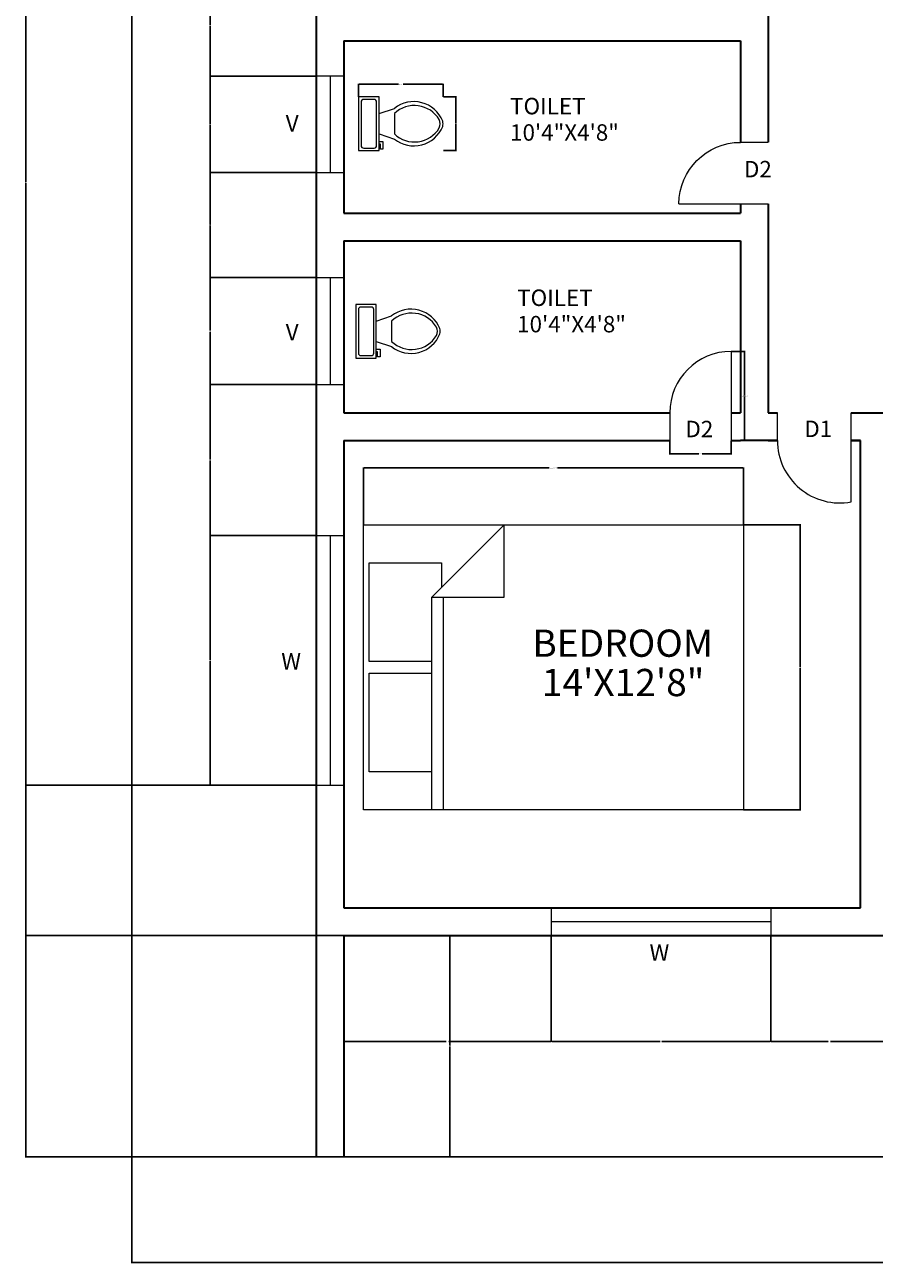
# Model space of a CAD drawing. Units: feet. Extents: x 1508 to 2265, y 1718 to 2421.
# Tile 1 of 4: x 1508 to 1784, y 1718 to 2121. Entities that reach past the tile are written whole.
import ezdxf

# ---------------------------------------------------------------- set-up
doc = ezdxf.new("R2010")
doc.units = ezdxf.units.FT
for name, color, linetype, lineweight in [('A-ANNO-DIMS', 2, 'Continuous', 18), ('A-ANNO-TEXT', 3, 'Continuous', 13), ('A-AREA-IDEN', 7, 'Continuous', 18), ('A-DOOR', 3, 'Continuous', 18), ('A-FLOR-FIXT', 9, 'Continuous', 18), ('A-FURN', 8, 'Continuous', 18), ('A-GLAZ', 4, 'Continuous', 18), ('A-WALL', 7, 'Continuous', 35), ('C-PROP', 7, 'Continuous', 25)]:
    doc.layers.add(name, color=color, linetype=linetype, lineweight=lineweight)
doc.styles.get("Standard").update_dxf_attribs({"font": 'arial.ttf'})
doc.dimstyles.get("Standard").update_dxf_attribs({"dimtxt": 0.18, "dimasz": 0.18, "dimexe": 0.18, "dimexo": 0.0625, "dimgap": 0.09, "dimtad": 0, "dimtih": 1, "dimtoh": 1, "dimdec": 4, "dimzin": 0, "dimdsep": 46, "dimtxsty": 'Standard', "dimcen": 0.09, "dimadec": 0, "dimazin": 0, "dimtfac": 1, "dimtdec": 4, "dimtofl": 0, "dimtmove": 0, "dimatfit": 3, "dimfxl": 1, "dimtolj": 1, "dimtzin": 0, "dimarcsym": 0})

# ---------------------------------------------------------------- blocks, each defined once
blk = doc.blocks.new('Toilet - top')
for p, q in [((9.5, -6), (9.5, -2)), ((-10, -8.5), (-8, -8.5)), ((-10, -9.5), (-10, -8.5)), ((-7, -9.5), (-10, -9.5)), ((-8, -8.5), (-8, -8)), ((-7, -8), (-7, -9.5)), ((-4, -8), (-6, -14)), ((4, -8), (6, -14)), ((4, -14), (-4, -14))]:
    blk.add_line(p, q)
blk.add_lwpolyline([(10.5, -8), (10.5, 0), (-10.5, 0), (-10.5, -8)], close=True)
for points in [[(-9.5, -2), (-9.5, -6)], [(8.5, -1), (-8.5, -1)], [(-8.5, -7), (8.5, -7)]]:
    blk.add_lwpolyline(points)
for centre, radius, start, end in [((-8.62, -1.88), 0.884, 81.8699, 188.1301), ((8.62, -1.88), 0.884, 351.8699, 98.1301), ((-8.62, -6.12), 0.884, 171.8699, 278.1301), ((8.62, -6.12), 0.884, 261.8699, 8.1301), ((3.52, -21.58), 12.17, 141.4691, 247.9714), ((4.2, -21.82), 11.33, 136.3677, 238.9468), ((-3.52, -21.58), 12.17, 292.0284, 38.5307), ((-4.2, -21.82), 11.33, 301.053, 43.6321), ((0, -27.88), 4, 245.7318, 294.2682), ((0, -29), 4, 254.8605, 285.1395)]:
    blk.add_arc(centre, radius, start, end)
blk = doc.blocks.new('Bed - Queen')
for p, q in [((0, -80.00003), (0, 0)), ((0, 0), (59.99999, 0)), ((59.99999, 0), (59.99999, -80.00003)), ((7.99999, -1.2), (28.79998, -1.2)), ((7.99999, -14.4), (7.99999, -1.2)), ((28.79998, -1.2), (28.79998, -14.4)), ((31.19999, -1.2), (51.99999, -1.2)), ((31.19999, -14.4), (31.19999, -1.2)), ((51.99999, -1.2), (51.99999, -16.4)), ((0, -14.4), (44.8, -14.4)), ((59.99999, -29.6), (44.8, -14.4)), ((44.8, -14.4), (44.8, -29.6)), ((44.8, -16.8), (0, -16.8)), ((51.99999, -16.4), (46.79936, -16.4)), ((44.8, -29.6), (59.99999, -29.6)), ((59.99999, -80.00003), (0, -80.00003))]:
    blk.add_line(p, q)
blk = doc.blocks.new('DOOR-LEAF-20')
blk.add_line((20, 29), (20, 0))
blk.add_arc((20, 9), 20, 90, 180)
blk = doc.blocks.new('*D13')
at = {"layer": 'A-ANNO-DIMS', "color": 0, "lineweight": -2, "transparency": 16777216}
for p, q in [((1737.87, 2014.26), (1742.33, 2014.26)), ((1742.15, 2014.08), (1742.15, 1999.94)), ((1742.15, 1985.44), (1742.15, 1999.58)), ((1737.87, 1985.26), (1742.33, 1985.26))]:
    blk.add_line(p, q, dxfattribs=at)
at = {"layer": 'A-ANNO-DIMS', "color": 0, "transparency": 16777216}
for points in [[(1742.12, 2014.08), (1742.18, 2014.08), (1742.15, 2014.26)], [(1742.12, 1985.44), (1742.18, 1985.44), (1742.15, 1985.26)]]:
    blk.add_solid(points, dxfattribs=at)
at = {"layer": 'Defpoints', "color": 0, "transparency": 16777216}
for p in [(1737.8, 2014.26), (1742.15, 2014.26), (1737.8, 1985.26)]:
    blk.add_point(p, dxfattribs=at)
at = {"layer": 'A-ANNO-DIMS', "color": 0, "transparency": 16777216, "insert": (1742.15, 1999.76), "char_height": 0.18, "attachment_point": 5}
blk.add_mtext('\\A1;D2 SWING 29 TYP.', dxfattribs=at)
blk = doc.blocks.new('*D14')
at = {"layer": 'A-ANNO-DIMS', "color": 0, "lineweight": -2, "transparency": 16777216}
for p, q in [((1717.8, 1985.2), (1717.8, 1980.73)), ((1737.8, 1985.2), (1737.8, 1980.73)), ((1717.98, 1980.91), (1727.28, 1980.91)), ((1737.62, 1980.91), (1728.33, 1980.91))]:
    blk.add_line(p, q, dxfattribs=at)
at = {"layer": 'A-ANNO-DIMS', "color": 0, "transparency": 16777216}
for points in [[(1717.98, 1980.94), (1717.98, 1980.88), (1717.8, 1980.91)], [(1737.62, 1980.94), (1737.62, 1980.88), (1737.8, 1980.91)]]:
    blk.add_solid(points, dxfattribs=at)
at = {"layer": 'Defpoints', "color": 0, "transparency": 16777216}
for p in [(1717.8, 1985.26), (1737.8, 1985.26), (1737.8, 1980.91)]:
    blk.add_point(p, dxfattribs=at)
at = {"layer": 'A-ANNO-DIMS', "color": 0, "transparency": 16777216, "insert": (1727.8, 1980.91), "char_height": 0.18, "attachment_point": 5}
blk.add_mtext('\\A1;20 TYP.', dxfattribs=at)
blk = doc.blocks.new('*D15')
at = {"layer": 'A-ANNO-DIMS', "color": 0, "lineweight": -2, "transparency": 16777216}
for p, q in [((1618.2, 1957.86), (1618.2, 1976.51)), ((1618.38, 1976.33), (1678.59, 1976.33)), ((1741.56, 1976.33), (1681.34, 1976.33)), ((1741.74, 1957.86), (1741.74, 1976.51))]:
    blk.add_line(p, q, dxfattribs=at)
at = {"layer": 'A-ANNO-DIMS', "color": 0, "transparency": 16777216}
for points in [[(1618.38, 1976.36), (1618.38, 1976.3), (1618.2, 1976.33)], [(1741.56, 1976.36), (1741.56, 1976.3), (1741.74, 1976.33)]]:
    blk.add_solid(points, dxfattribs=at)
at = {"layer": 'Defpoints', "color": 0, "transparency": 16777216}
for p in [(1618.2, 1976.33), (1618.2, 1957.8), (1741.74, 1957.8)]:
    blk.add_point(p, dxfattribs=at)
at = {"layer": 'A-ANNO-DIMS', "color": 0, "transparency": 16777216, "insert": (1679.97, 1976.33), "char_height": 0.18, "attachment_point": 5}
blk.add_mtext('\\A1;QUEEN BED 124 TYP.', dxfattribs=at)
blk = doc.blocks.new('*D16')
at = {"layer": 'A-ANNO-DIMS', "color": 0, "lineweight": -2, "transparency": 16777216}
for p, q in [((1741.8, 1957.8), (1760.45, 1957.8)), ((1760.27, 1957.62), (1760.27, 1911.65)), ((1760.27, 1865.32), (1760.27, 1911.29)), ((1741.8, 1865.14), (1760.45, 1865.14))]:
    blk.add_line(p, q, dxfattribs=at)
at = {"layer": 'A-ANNO-DIMS', "color": 0, "transparency": 16777216}
for points in [[(1760.24, 1957.62), (1760.3, 1957.62), (1760.27, 1957.8)], [(1760.24, 1865.32), (1760.3, 1865.32), (1760.27, 1865.14)]]:
    blk.add_solid(points, dxfattribs=at)
at = {"layer": 'Defpoints', "color": 0, "transparency": 16777216}
for p in [(1741.74, 1957.8), (1760.27, 1957.8), (1741.74, 1865.14)]:
    blk.add_point(p, dxfattribs=at)
at = {"layer": 'A-ANNO-DIMS', "color": 0, "transparency": 16777216, "insert": (1760.27, 1911.47), "char_height": 0.18, "attachment_point": 5}
blk.add_mtext('\\A1;93 TYP.', dxfattribs=at)
blk = doc.blocks.new('*D17')
at = {"layer": 'A-ANNO-DIMS', "color": 0, "lineweight": -2, "transparency": 16777216}
for p, q in [((1616.62, 2097.09), (1616.62, 2101.33)), ((1616.8, 2101.15), (1629.58, 2101.15)), ((1643.92, 2101.15), (1631.14, 2101.15)), ((1644.1, 2097.09), (1644.1, 2101.33))]:
    blk.add_line(p, q, dxfattribs=at)
at = {"layer": 'A-ANNO-DIMS', "color": 0, "transparency": 16777216}
for points in [[(1616.8, 2101.18), (1616.8, 2101.12), (1616.62, 2101.15)], [(1643.92, 2101.18), (1643.92, 2101.12), (1644.1, 2101.15)]]:
    blk.add_solid(points, dxfattribs=at)
at = {"layer": 'Defpoints', "color": 0, "transparency": 16777216}
for p in [(1616.62, 2101.15), (1616.62, 2097.03), (1644.1, 2097.03)]:
    blk.add_point(p, dxfattribs=at)
at = {"layer": 'A-ANNO-DIMS', "color": 0, "transparency": 16777216, "insert": (1630.36, 2101.15), "char_height": 0.18, "attachment_point": 5}
blk.add_mtext('\\A1;WC 27 TYP.', dxfattribs=at)
blk = doc.blocks.new('*D18')
at = {"layer": 'A-ANNO-DIMS', "color": 0, "lineweight": -2, "transparency": 16777216}
for p, q in [((1644.16, 2097.03), (1648.4, 2097.03)), ((1648.22, 2096.85), (1648.22, 2088.48)), ((1648.22, 2079.75), (1648.22, 2088.12)), ((1644.16, 2079.57), (1648.4, 2079.57))]:
    blk.add_line(p, q, dxfattribs=at)
at = {"layer": 'A-ANNO-DIMS', "color": 0, "transparency": 16777216}
for points in [[(1648.19, 2096.85), (1648.25, 2096.85), (1648.22, 2097.03)], [(1648.19, 2079.75), (1648.25, 2079.75), (1648.22, 2079.57)]]:
    blk.add_solid(points, dxfattribs=at)
at = {"layer": 'Defpoints', "color": 0, "transparency": 16777216}
for p in [(1644.1, 2097.03), (1648.22, 2097.03), (1644.1, 2079.57)]:
    blk.add_point(p, dxfattribs=at)
at = {"layer": 'A-ANNO-DIMS', "color": 0, "transparency": 16777216, "insert": (1648.22, 2088.3), "char_height": 0.18, "attachment_point": 5}
blk.add_mtext('\\A1;17 TYP.', dxfattribs=at)
blk = doc.blocks.new('*D31')
at = {"layer": 'A-ANNO-DIMS', "color": 0, "lineweight": -2, "transparency": 16777216}
for p, q in [((1542.8, 1752.2), (1542.8, 1717.61)), ((2230.8, 1752.2), (2230.8, 1717.61)), ((1542.98, 1717.79), (1886.52, 1717.79)), ((2230.62, 1717.79), (1887.09, 1717.79))]:
    blk.add_line(p, q, dxfattribs=at)
at = {"layer": 'A-ANNO-DIMS', "color": 0, "transparency": 16777216}
for points in [[(1542.98, 1717.82), (1542.98, 1717.76), (1542.8, 1717.79)], [(2230.62, 1717.82), (2230.62, 1717.76), (2230.8, 1717.79)]]:
    blk.add_solid(points, dxfattribs=at)
at = {"layer": 'Defpoints', "color": 0, "transparency": 16777216}
for p in [(1542.8, 1752.26), (2230.8, 1752.26), (2230.8, 1717.79)]:
    blk.add_point(p, dxfattribs=at)
at = {"layer": 'A-ANNO-DIMS', "color": 0, "transparency": 16777216, "insert": (1886.8, 1717.79), "char_height": 0.18, "attachment_point": 5}
blk.add_mtext('\\A1;688', dxfattribs=at)
blk = doc.blocks.new('*D32')
at = {"layer": 'A-ANNO-DIMS', "color": 0, "lineweight": -2, "transparency": 16777216}
for p, q in [((1542.74, 2386.26), (1508.15, 2386.26)), ((1508.33, 2386.08), (1508.33, 2069.44)), ((1508.33, 1752.44), (1508.33, 2069.08)), ((1542.74, 1752.26), (1508.15, 1752.26))]:
    blk.add_line(p, q, dxfattribs=at)
at = {"layer": 'A-ANNO-DIMS', "color": 0, "transparency": 16777216}
for points in [[(1508.3, 2386.08), (1508.36, 2386.08), (1508.33, 2386.26)], [(1508.3, 1752.44), (1508.36, 1752.44), (1508.33, 1752.26)]]:
    blk.add_solid(points, dxfattribs=at)
at = {"layer": 'Defpoints', "color": 0, "transparency": 16777216}
for p in [(1508.33, 2386.26), (1542.8, 2386.26), (1542.8, 1752.26)]:
    blk.add_point(p, dxfattribs=at)
at = {"layer": 'A-ANNO-DIMS', "color": 0, "transparency": 16777216, "insert": (1508.33, 2069.26), "char_height": 0.18, "attachment_point": 5}
blk.add_mtext('\\A1;634', dxfattribs=at)
blk = doc.blocks.new('*D35')
at = {"layer": 'A-ANNO-DIMS', "color": 0, "lineweight": -2, "transparency": 16777216}
for p, q in [((1611.87, 1824.26), (1646.46, 1824.26)), ((1646.28, 1824.08), (1646.28, 1788.44)), ((1646.28, 1752.44), (1646.28, 1788.08)), ((1611.87, 1752.26), (1646.46, 1752.26))]:
    blk.add_line(p, q, dxfattribs=at)
at = {"layer": 'A-ANNO-DIMS', "color": 0, "transparency": 16777216}
for points in [[(1646.25, 1824.08), (1646.31, 1824.08), (1646.28, 1824.26)], [(1646.25, 1752.44), (1646.31, 1752.44), (1646.28, 1752.26)]]:
    blk.add_solid(points, dxfattribs=at)
at = {"layer": 'Defpoints', "color": 0, "transparency": 16777216}
for p in [(1611.8, 1824.26), (1611.8, 1752.26), (1646.28, 1752.26)]:
    blk.add_point(p, dxfattribs=at)
at = {"layer": 'A-ANNO-DIMS', "color": 0, "transparency": 16777216, "insert": (1646.28, 1788.26), "char_height": 0.18, "attachment_point": 5}
blk.add_mtext('\\A1;72', dxfattribs=at)
blk = doc.blocks.new('*D53')
at = {"layer": 'A-ANNO-DIMS', "color": 0, "lineweight": -2, "transparency": 16777216}
for p, q in [((1602.74, 1873.09), (1508.15, 1873.09)), ((1508.33, 1872.91), (1508.33, 1848.86)), ((1508.33, 1824.44), (1508.33, 1848.49)), ((1611.74, 1824.26), (1508.15, 1824.26))]:
    blk.add_line(p, q, dxfattribs=at)
at = {"layer": 'A-ANNO-DIMS', "color": 0, "transparency": 16777216}
for points in [[(1508.3, 1872.91), (1508.36, 1872.91), (1508.33, 1873.09)], [(1508.3, 1824.44), (1508.36, 1824.44), (1508.33, 1824.26)]]:
    blk.add_solid(points, dxfattribs=at)
at = {"layer": 'Defpoints', "color": 0, "transparency": 16777216}
for p in [(1508.33, 1873.09), (1602.8, 1873.09), (1611.8, 1824.26)]:
    blk.add_point(p, dxfattribs=at)
at = {"layer": 'A-ANNO-DIMS', "color": 0, "transparency": 16777216, "insert": (1508.33, 1848.67), "char_height": 0.18, "attachment_point": 5}
blk.add_mtext('\\A1;48.83', dxfattribs=at)
blk = doc.blocks.new('*D54')
at = {"layer": 'A-ANNO-DIMS', "color": 0, "lineweight": -2, "transparency": 16777216}
for p, q in [((1602.74, 1954.4), (1568.15, 1954.4)), ((1568.33, 1954.22), (1568.33, 1913.93)), ((1568.33, 1873.27), (1568.33, 1913.56)), ((1602.74, 1873.09), (1568.15, 1873.09))]:
    blk.add_line(p, q, dxfattribs=at)
at = {"layer": 'A-ANNO-DIMS', "color": 0, "transparency": 16777216}
for points in [[(1568.3, 1954.22), (1568.36, 1954.22), (1568.33, 1954.4)], [(1568.3, 1873.27), (1568.36, 1873.27), (1568.33, 1873.09)]]:
    blk.add_solid(points, dxfattribs=at)
at = {"layer": 'Defpoints', "color": 0, "transparency": 16777216}
for p in [(1568.33, 1954.4), (1602.8, 1954.4), (1602.8, 1873.09)]:
    blk.add_point(p, dxfattribs=at)
at = {"layer": 'A-ANNO-DIMS', "color": 0, "transparency": 16777216, "insert": (1568.33, 1913.75), "char_height": 0.18, "attachment_point": 5}
blk.add_mtext('\\A1;81.32', dxfattribs=at)
blk = doc.blocks.new('*D55')
at = {"layer": 'A-ANNO-DIMS', "color": 0, "lineweight": -2, "transparency": 16777216}
for p, q in [((1602.74, 2003.44), (1568.15, 2003.44)), ((1568.33, 2003.26), (1568.33, 1979.11)), ((1568.33, 1954.58), (1568.33, 1978.74)), ((1602.74, 1954.4), (1568.15, 1954.4))]:
    blk.add_line(p, q, dxfattribs=at)
at = {"layer": 'A-ANNO-DIMS', "color": 0, "transparency": 16777216}
for points in [[(1568.3, 2003.26), (1568.36, 2003.26), (1568.33, 2003.44)], [(1568.3, 1954.58), (1568.36, 1954.58), (1568.33, 1954.4)]]:
    blk.add_solid(points, dxfattribs=at)
at = {"layer": 'Defpoints', "color": 0, "transparency": 16777216}
for p in [(1568.33, 2003.44), (1602.8, 2003.44), (1602.8, 1954.4)]:
    blk.add_point(p, dxfattribs=at)
at = {"layer": 'A-ANNO-DIMS', "color": 0, "transparency": 16777216, "insert": (1568.33, 1978.92), "char_height": 0.18, "attachment_point": 5}
blk.add_mtext('\\A1;49.04', dxfattribs=at)
blk = doc.blocks.new('*D56')
at = {"layer": 'A-ANNO-DIMS', "color": 0, "lineweight": -2, "transparency": 16777216}
for p, q in [((1602.74, 2038.25), (1568.15, 2038.25)), ((1568.33, 2038.07), (1568.33, 2021.03)), ((1568.33, 2003.62), (1568.33, 2020.66)), ((1602.74, 2003.44), (1568.15, 2003.44))]:
    blk.add_line(p, q, dxfattribs=at)
at = {"layer": 'A-ANNO-DIMS', "color": 0, "transparency": 16777216}
for points in [[(1568.3, 2038.07), (1568.36, 2038.07), (1568.33, 2038.25)], [(1568.3, 2003.62), (1568.36, 2003.62), (1568.33, 2003.44)]]:
    blk.add_solid(points, dxfattribs=at)
at = {"layer": 'Defpoints', "color": 0, "transparency": 16777216}
for p in [(1568.33, 2038.25), (1602.8, 2038.25), (1602.8, 2003.44)]:
    blk.add_point(p, dxfattribs=at)
at = {"layer": 'A-ANNO-DIMS', "color": 0, "transparency": 16777216, "insert": (1568.33, 2020.84), "char_height": 0.18, "attachment_point": 5}
blk.add_mtext('\\A1;34.804', dxfattribs=at)
blk = doc.blocks.new('*D57')
at = {"layer": 'A-ANNO-DIMS', "color": 0, "lineweight": -2, "transparency": 16777216}
for p, q in [((1602.74, 2072.43), (1568.15, 2072.43)), ((1568.33, 2072.25), (1568.33, 2055.52)), ((1568.33, 2038.43), (1568.33, 2055.16)), ((1602.74, 2038.25), (1568.15, 2038.25))]:
    blk.add_line(p, q, dxfattribs=at)
at = {"layer": 'A-ANNO-DIMS', "color": 0, "transparency": 16777216}
for points in [[(1568.3, 2072.25), (1568.36, 2072.25), (1568.33, 2072.43)], [(1568.3, 2038.43), (1568.36, 2038.43), (1568.33, 2038.25)]]:
    blk.add_solid(points, dxfattribs=at)
at = {"layer": 'Defpoints', "color": 0, "transparency": 16777216}
for p in [(1568.33, 2072.43), (1602.8, 2072.43), (1602.8, 2038.25)]:
    blk.add_point(p, dxfattribs=at)
at = {"layer": 'A-ANNO-DIMS', "color": 0, "transparency": 16777216, "insert": (1568.33, 2055.34), "char_height": 0.18, "attachment_point": 5}
blk.add_mtext('\\A1;34.19', dxfattribs=at)
blk = doc.blocks.new('*D58')
at = {"layer": 'A-ANNO-DIMS', "color": 0, "lineweight": -2, "transparency": 16777216}
for p, q in [((1602.74, 2103.84), (1568.15, 2103.84)), ((1568.33, 2103.66), (1568.33, 2088.32)), ((1568.33, 2072.61), (1568.33, 2087.96)), ((1602.74, 2072.43), (1568.15, 2072.43))]:
    blk.add_line(p, q, dxfattribs=at)
at = {"layer": 'A-ANNO-DIMS', "color": 0, "transparency": 16777216}
for points in [[(1568.3, 2103.66), (1568.36, 2103.66), (1568.33, 2103.84)], [(1568.3, 2072.61), (1568.36, 2072.61), (1568.33, 2072.43)]]:
    blk.add_solid(points, dxfattribs=at)
at = {"layer": 'Defpoints', "color": 0, "transparency": 16777216}
for p in [(1568.33, 2103.84), (1602.8, 2103.84), (1602.8, 2072.43)]:
    blk.add_point(p, dxfattribs=at)
at = {"layer": 'A-ANNO-DIMS', "color": 0, "transparency": 16777216, "insert": (1568.33, 2088.14), "char_height": 0.18, "attachment_point": 5}
blk.add_mtext('\\A1;31.41', dxfattribs=at)
blk = doc.blocks.new('*D59')
at = {"layer": 'A-ANNO-DIMS', "color": 0, "lineweight": -2, "transparency": 16777216}
for p, q in [((1602.74, 2136.59), (1568.15, 2136.59)), ((1568.33, 2136.41), (1568.33, 2120.4)), ((1568.33, 2104.02), (1568.33, 2120.03)), ((1602.74, 2103.84), (1568.15, 2103.84))]:
    blk.add_line(p, q, dxfattribs=at)
at = {"layer": 'A-ANNO-DIMS', "color": 0, "transparency": 16777216}
for points in [[(1568.3, 2136.41), (1568.36, 2136.41), (1568.33, 2136.59)], [(1568.3, 2104.02), (1568.36, 2104.02), (1568.33, 2103.84)]]:
    blk.add_solid(points, dxfattribs=at)
at = {"layer": 'Defpoints', "color": 0, "transparency": 16777216}
for p in [(1568.33, 2136.59), (1602.8, 2136.59), (1602.8, 2103.84)]:
    blk.add_point(p, dxfattribs=at)
at = {"layer": 'A-ANNO-DIMS', "color": 0, "transparency": 16777216, "insert": (1568.33, 2120.22), "char_height": 0.18, "attachment_point": 5}
blk.add_mtext('\\A1;32.74', dxfattribs=at)
blk = doc.blocks.new('*D66')
at = {"layer": 'A-ANNO-DIMS', "color": 0, "lineweight": -2, "transparency": 16777216}
for p, q in [((1611.8, 1824.2), (1611.8, 1789.61)), ((1679.25, 1824.2), (1679.25, 1789.61)), ((1611.98, 1789.79), (1645.13, 1789.79)), ((1679.07, 1789.79), (1645.92, 1789.79))]:
    blk.add_line(p, q, dxfattribs=at)
at = {"layer": 'A-ANNO-DIMS', "color": 0, "transparency": 16777216}
for points in [[(1611.98, 1789.82), (1611.98, 1789.76), (1611.8, 1789.79)], [(1679.07, 1789.82), (1679.07, 1789.76), (1679.25, 1789.79)]]:
    blk.add_solid(points, dxfattribs=at)
at = {"layer": 'Defpoints', "color": 0, "transparency": 16777216}
for p in [(1611.8, 1824.26), (1679.25, 1824.26), (1611.8, 1789.79)]:
    blk.add_point(p, dxfattribs=at)
at = {"layer": 'A-ANNO-DIMS', "color": 0, "transparency": 16777216, "insert": (1645.53, 1789.79), "char_height": 0.18, "attachment_point": 5}
blk.add_mtext('\\A1;67.45', dxfattribs=at)
blk = doc.blocks.new('*D67')
at = {"layer": 'A-ANNO-DIMS', "color": 0, "lineweight": -2, "transparency": 16777216}
for p, q in [((1679.25, 1824.2), (1679.25, 1789.61)), ((1750.65, 1824.2), (1750.65, 1789.61)), ((1679.43, 1789.79), (1714.63, 1789.79)), ((1750.47, 1789.79), (1715.27, 1789.79))]:
    blk.add_line(p, q, dxfattribs=at)
at = {"layer": 'A-ANNO-DIMS', "color": 0, "transparency": 16777216}
for points in [[(1679.43, 1789.82), (1679.43, 1789.76), (1679.25, 1789.79)], [(1750.47, 1789.82), (1750.47, 1789.76), (1750.65, 1789.79)]]:
    blk.add_solid(points, dxfattribs=at)
at = {"layer": 'Defpoints', "color": 0, "transparency": 16777216}
for p in [(1679.25, 1824.26), (1750.65, 1824.26), (1679.25, 1789.79)]:
    blk.add_point(p, dxfattribs=at)
at = {"layer": 'A-ANNO-DIMS', "color": 0, "transparency": 16777216, "insert": (1714.95, 1789.79), "char_height": 0.18, "attachment_point": 5}
blk.add_mtext('\\A1;71.4', dxfattribs=at)
blk = doc.blocks.new('*D68')
at = {"layer": 'A-ANNO-DIMS', "color": 0, "lineweight": -2, "transparency": 16777216}
for p, q in [((1750.65, 1824.2), (1750.65, 1789.61)), ((1788.8, 1824.2), (1788.8, 1789.61)), ((1750.83, 1789.79), (1769.33, 1789.79)), ((1788.62, 1789.79), (1770.12, 1789.79))]:
    blk.add_line(p, q, dxfattribs=at)
at = {"layer": 'A-ANNO-DIMS', "color": 0, "transparency": 16777216}
for points in [[(1750.83, 1789.82), (1750.83, 1789.76), (1750.65, 1789.79)], [(1788.62, 1789.82), (1788.62, 1789.76), (1788.8, 1789.79)]]:
    blk.add_solid(points, dxfattribs=at)
at = {"layer": 'Defpoints', "color": 0, "transparency": 16777216}
for p in [(1750.65, 1824.26), (1788.8, 1824.26), (1750.65, 1789.79)]:
    blk.add_point(p, dxfattribs=at)
at = {"layer": 'A-ANNO-DIMS', "color": 0, "transparency": 16777216, "insert": (1769.73, 1789.79), "char_height": 0.18, "attachment_point": 5}
blk.add_mtext('\\A1;38.15', dxfattribs=at)

msp = doc.modelspace()

# ---------------------------------------------------------------- linework, layer by layer
at = {"layer": 'A-DOOR'}
for p, q in [((1740.8049, 2082.2608), (1749.8049, 2082.2608)), ((1717.8049, 1994.2608), (1717.8049, 1985.2608)), ((1752.8049, 1985.2608), (1752.8049, 1994.2608)), ((1776.8049, 1965.2608), (1776.8049, 1994.2608))]:
    msp.add_line(p, q, dxfattribs=at)
msp.add_arc((1773.1382, 1985.2608), 20.3333, 180, 280.388858, dxfattribs=at)
at = {"layer": 'A-GLAZ'}
for p, q in [((1602.8049, 2103.8448), (1611.8049, 2103.8448)), ((1607.3049, 2103.8448), (1607.3049, 2072.4348)), ((1602.8049, 2072.4348), (1611.8049, 2072.4348)), ((1602.8049, 2038.2467), (1611.8049, 2038.2467)), ((1607.3049, 2038.2467), (1607.3049, 2003.4426)), ((1602.8049, 2003.4426), (1611.8049, 2003.4426)), ((1602.8049, 1954.4046), (1611.8049, 1954.4046)), ((1607.3049, 1954.4046), (1607.3049, 1873.0878)), ((1602.8049, 1873.0878), (1611.8049, 1873.0878)), ((1679.2508, 1833.2608), (1679.2508, 1824.2608)), ((1750.6528, 1833.2608), (1750.6528, 1824.2608)), ((1679.2508, 1828.7608), (1750.6528, 1828.7608))]:
    msp.add_line(p, q, dxfattribs=at)
at = {"layer": 'A-WALL'}
for p, q in [((1602.8049, 2192.2608), (1602.8049, 1752.2608)), ((1749.8049, 2189.2608), (1749.8049, 2082.2608)), ((1602.8049, 2115.2608), (1602.8049, 2059.2608)), ((1611.8049, 2115.2608), (1740.8049, 2115.2608)), ((1611.8049, 2115.2608), (1611.8049, 2059.2608)), ((1680.8049, 2115.2608), (1740.8049, 2115.2608)), ((1740.8049, 2115.2608), (1740.8049, 2082.2608)), ((1611.8049, 2059.2608), (1740.8049, 2059.2608)), ((1740.8049, 2062.2608), (1740.8049, 2059.2608)), ((1749.8049, 2062.2608), (1749.8049, 1994.2608)), ((1602.8049, 2050.2608), (1602.8049, 1994.2608)), ((1611.8049, 2050.2608), (1740.8049, 2050.2608)), ((1611.8049, 2050.2608), (1611.8049, 1994.2608)), ((1740.8049, 2050.2608), (1740.8049, 1994.2608)), ((1611.8049, 1994.2608), (1717.8049, 1994.2608)), ((1737.8049, 1994.2608), (1740.8049, 1994.2608)), ((1749.8049, 1994.2608), (1752.8049, 1994.2608)), ((1776.8049, 1994.2608), (1791.8049, 1994.2608)), ((1602.8049, 1985.2608), (1602.8049, 1752.2608)), ((1611.8049, 1985.2608), (1717.8049, 1985.2608)), ((1611.8049, 1985.2608), (1611.8049, 1833.2608)), ((1737.8049, 1985.2608), (1740.8049, 1985.2608)), ((1752.8049, 1985.2608), (1740.8049, 1985.2608)), ((1749.8049, 1985.2608), (1752.8049, 1985.2608)), ((1779.8049, 1985.2608), (1776.8049, 1985.2608)), ((1776.8049, 1985.2608), (1779.8049, 1985.2608)), ((1779.8049, 1833.2608), (1779.8049, 1985.2608)), ((1611.8049, 1833.2608), (1779.8049, 1833.2608)), ((1611.8049, 1824.2608), (1974.8049, 1824.2608)), ((1611.8049, 1824.2608), (1611.8049, 1752.2608))]:
    msp.add_line(p, q, dxfattribs=at)
at = {"layer": 'C-PROP'}
for p, q in [((1542.8049, 2386.2608), (1542.8049, 1752.2608)), ((1602.8049, 1752.2608), (1542.8049, 1752.2608)), ((1611.8049, 1752.2608), (1602.8049, 1752.2608)), ((1611.8049, 1752.2608), (2230.8049, 1752.2608))]:
    msp.add_line(p, q, dxfattribs=at)

# ---------------------------------------------------------------- block references
at = {"layer": 'A-DOOR', "extrusion": (0, 0, -1), "zscale": -1, "rotation": 270.0000000000007}
msp.add_blockref('DOOR-LEAF-20', (-1749.8046, 2082.2606), dxfattribs=at)
at = {"layer": 'A-DOOR'}
msp.add_blockref('DOOR-LEAF-20', (1717.805, 1985.261), dxfattribs=at)
at = {"layer": 'A-FLOR-FIXT', "xscale": 0.8315942650714294, "yscale": 0.8315942650714294, "zscale": 0.8315942650714294, "rotation": 90}
for p in [(1616.6188, 2088.2998), (1615.7002, 2020.784)]:
    msp.add_blockref('Toilet - top', p, dxfattribs=at)
at = {"layer": 'A-FURN', "xscale": 1.544203597856591, "yscale": 1.544203597856591, "zscale": 1.544203597856591, "rotation": 90}
msp.add_blockref('Bed - Queen', (1618.1998, 1865.1449), dxfattribs=at)

# ---------------------------------------------------------------- texts
at = {"layer": 'A-ANNO-TEXT'}
for s, height, p in [('V', 5.3453, (1592.8942, 2085.7633)), ('D2', 5.34528, (1741.9372, 2070.8617)), ('V', 5.3453, (1592.8942, 2017.8526)), ('D2', 5.34528, (1722.8941, 1986.3233)), ('D1', 5.34528, (1761.5653, 1986.3768)), ('W', 5.3453, (1591.4512, 1910.7582)), ('W', 5.3453, (1711.2296, 1815.9883))]:
    msp.add_text(s, height=height, dxfattribs=at).set_placement(p)
at = {"layer": 'A-AREA-IDEN'}
for s, height, p in [('TOILET', 5.34528, (1665.8694, 2091.3765)), ('10\'4"X4\'8"', 5.34528, (1665.8694, 2082.7898)), ('TOILET', 5.34528, (1668.1636, 2029.0268)), ('10\'4"X4\'8"', 5.34528, (1668.1636, 2020.4401)), ('BEDROOM', 8.85057, (1673.1135, 1914.8931)), ('14\'X12\'8"', 8.85057, (1676.1992, 1902.1022))]:
    msp.add_text(s, height=height, dxfattribs=at).set_placement(p)

# ---------------------------------------------------------------- dimensions: what is measured, and where the dimension line sits
at = {"layer": 'A-ANNO-DIMS'}
for base, p1, p2, angle, override, picture, middle in [((1508.3299, 2386.2608), (1542.8049, 1752.2608), (1542.8049, 2386.2608), 90, {"dimdec": 0, "dimlfac": 1, "dimrnd": 0, "dimzin": 0, "dimdsep": 46, "dimlunit": 2}, '*D32', (1508.3299, 2069.2608)), ((1568.3299, 2136.588), (1602.8049, 2103.8448), (1602.8049, 2136.588), 90, {"dimdec": 2, "dimlfac": 1, "dimrnd": 0, "dimzin": 0, "dimdsep": 46, "dimlunit": 2}, '*D59', (1568.3299, 2120.2164)), ((1568.3299, 2103.8448), (1602.8049, 2072.4348), (1602.8049, 2103.8448), 90, {"dimdec": 2, "dimlfac": 1, "dimrnd": 0, "dimzin": 0, "dimdsep": 46, "dimlunit": 2}, '*D58', (1568.3299, 2088.1398)), ((1568.3299, 2072.4348), (1602.8049, 2038.2467), (1602.8049, 2072.4348), 90, {"dimdec": 2, "dimlfac": 1, "dimrnd": 0, "dimzin": 0, "dimdsep": 46, "dimlunit": 2}, '*D57', (1568.3299, 2055.3408)), ((1568.3299, 2038.2467), (1602.8049, 2003.4426), (1602.8049, 2038.2467), 90, {"dimdec": 3, "dimlfac": 1, "dimrnd": 0, "dimzin": 0, "dimdsep": 46, "dimlunit": 2}, '*D56', (1568.3299, 2020.8446)), ((1568.3299, 2003.4426), (1602.8049, 1954.4046), (1602.8049, 2003.4426), 90, {"dimdec": 2, "dimlfac": 1, "dimrnd": 0, "dimzin": 0, "dimdsep": 46, "dimlunit": 2}, '*D55', (1568.3299, 1978.9236)), ((1568.3299, 1954.4046), (1602.8049, 1873.0878), (1602.8049, 1954.4046), 90, {"dimdec": 2, "dimlfac": 1, "dimrnd": 0, "dimzin": 0, "dimdsep": 46, "dimlunit": 2}, '*D54', (1568.3299, 1913.7462)), ((1508.3299, 1873.0878), (1611.8049, 1824.2608), (1602.8049, 1873.0878), 90, {"dimdec": 2, "dimlfac": 1, "dimrnd": 0, "dimzin": 0, "dimdsep": 46, "dimlunit": 2}, '*D53', (1508.3299, 1848.6743)), ((1646.2799, 1752.2608), (1611.8049, 1824.2608), (1611.8049, 1752.2608), 270, {"dimdec": 0, "dimlfac": 1, "dimrnd": 0, "dimzin": 0, "dimdsep": 46, "dimlunit": 2}, '*D35', (1646.2799, 1788.2608)), ((1611.8049, 1789.7858), (1679.2508, 1824.2608), (1611.8049, 1824.2608), 180, {"dimdec": 2, "dimlfac": 1, "dimrnd": 0, "dimzin": 0, "dimdsep": 46, "dimlunit": 2}, '*D66', (1645.5278, 1789.7858)), ((1679.2508, 1789.7858), (1750.6528, 1824.2608), (1679.2508, 1824.2608), 180, {"dimdec": 1, "dimlfac": 1, "dimrnd": 0, "dimzin": 0, "dimdsep": 46, "dimlunit": 2}, '*D67', (1714.9518, 1789.7858)), ((1750.6528, 1789.7858), (1788.8049, 1824.2608), (1750.6528, 1824.2608), 180, {"dimdec": 2, "dimlfac": 1, "dimrnd": 0, "dimzin": 0, "dimdsep": 46, "dimlunit": 2}, '*D68', (1769.7289, 1789.7858))]:
    dim = msp.add_linear_dim(base=base, p1=p1, p2=p2, angle=angle, dimstyle='Standard', override=override, dxfattribs=at)
    dim.commit()
    dim.dimension.update_dxf_attribs({"geometry": picture, "text_midpoint": middle})
for base, p1, p2, angle, text, picture, middle in [((1616.6188, 2101.1537), (1644.0999, 2097.0315), (1616.6188, 2097.0315), 180, 'WC <> TYP.', '*D17', (1630.3593, 2101.1537)), ((1648.222, 2097.0315), (1644.0999, 2079.5681), (1644.0999, 2097.0315), 90, '<> TYP.', '*D18', (1648.222, 2088.2998)), ((1742.1549, 2014.2608), (1737.8049, 1985.2608), (1737.8049, 2014.2608), 90, 'D2 SWING <> TYP.', '*D13', (1742.1549, 1999.7608)), ((1618.1998, 1976.3275), (1741.7362, 1957.7971), (1618.1998, 1957.7971), 180, 'QUEEN BED <> TYP.', '*D15', (1679.968, 1976.3275)), ((1760.2666, 1957.7971), (1741.7362, 1865.1449), (1741.7362, 1957.7971), 90, '<> TYP.', '*D16', (1760.2666, 1911.471))]:
    dim = msp.add_linear_dim(base=base, p1=p1, p2=p2, angle=angle, text=text, dimstyle='Standard', override={"dimdec": 0, "dimlfac": 1, "dimrnd": 0, "dimzin": 0, "dimdsep": 46, "dimlunit": 2}, dxfattribs=at)
    dim.commit()
    dim.dimension.update_dxf_attribs({"geometry": picture, "text_midpoint": middle})
dim = msp.add_linear_dim(base=(1737.8049, 1980.9108), p1=(1717.8049, 1985.2608), p2=(1737.8049, 1985.2608), text='<> TYP.', dimstyle='Standard', override={"dimdec": 0, "dimlfac": 1, "dimrnd": 0, "dimzin": 0, "dimdsep": 46, "dimlunit": 2}, dxfattribs=at)
dim.commit()
dim.dimension.update_dxf_attribs({"geometry": '*D14', "text_midpoint": (1727.8049, 1980.9108)})
dim = msp.add_linear_dim(base=(2230.8049, 1717.7858), p1=(1542.8049, 1752.2608), p2=(2230.8049, 1752.2608), dimstyle='Standard', override={"dimdec": 0, "dimlfac": 1, "dimrnd": 0, "dimzin": 0, "dimdsep": 46, "dimlunit": 2}, dxfattribs=at)
dim.commit()
dim.dimension.update_dxf_attribs({"geometry": '*D31', "text_midpoint": (1886.8049, 1717.7858)})

doc.saveas('drawing.dxf')
